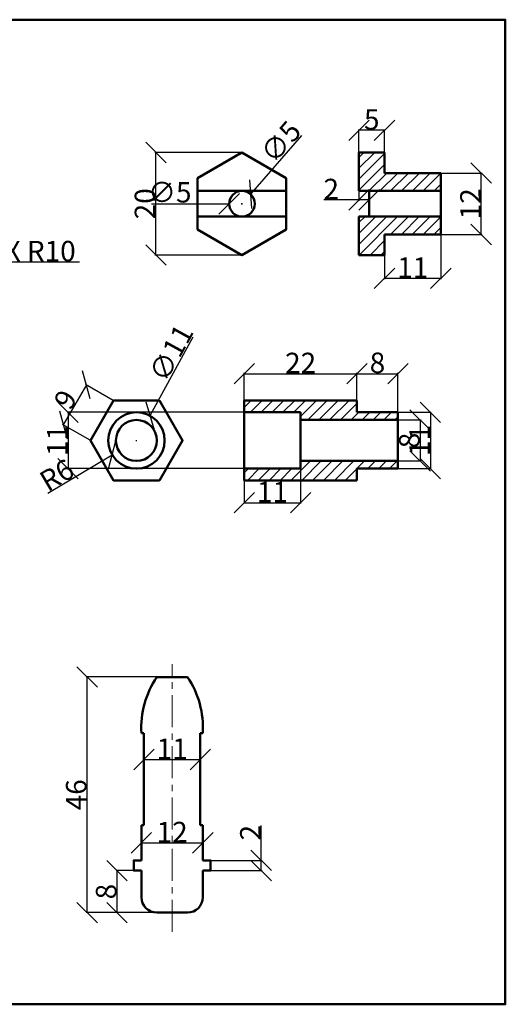
# Model space of a CAD drawing. Units: millimetres. Extents: x 4 to 224, y 3 to 195.
# Tile 2 of 2: x 129 to 224, y 3 to 195. Entities that reach past the tile are written whole.
import ezdxf

# ---------------------------------------------------------------- set-up
doc = ezdxf.new("R2010")
doc.units = ezdxf.units.MM
doc.header["$MEASUREMENT"] = 0
doc.linetypes.add('CENTER', pattern=[2, 1.25, -0.25, 0.25, -0.25])
for name, color, linetype, lineweight in [('M-CNTR', 1, 'CENTER', 18), ('M-DIMS', 2, 'Continuous', 25), ('M-HATC', 8, 'Continuous', 18), ('M-OUTL', 7, 'Continuous', 50)]:
    doc.layers.add(name, color=color, linetype=linetype, lineweight=lineweight)
doc.styles.get("Standard").update_dxf_attribs({"font": 'arial.ttf'})
doc.dimstyles.get("Standard").update_dxf_attribs({"dimtxt": 4, "dimasz": 4, "dimexe": 0.18, "dimexo": 0.0625, "dimgap": 0.09, "dimtad": 1, "dimdec": 0, "dimzin": 0, "dimdsep": 46, "dimtxsty": 'Standard', "dimblk": 'OBLIQUE', "dimcen": 0.09, "dimclre": 251, "dimadec": 0, "dimazin": 0, "dimtfac": 1, "dimtdec": 0, "dimtofl": 0, "dimtmove": 0, "dimatfit": 3, "dimfxl": 1, "dimtolj": 1, "dimtzin": 0, "dimarcsym": 0})

# ---------------------------------------------------------------- blocks, each defined once
blk = doc.blocks.new('_Oblique')
at = {"color": 0, "linetype": 'ByBlock', "lineweight": -2}
blk.add_line((-0.5, -0.5), (0.5, 0.5), dxfattribs=at)
blk = doc.blocks.new('*D10')
at = {"layer": 'Defpoints', "color": 0, "transparency": 16777216}
for p in [(156.03, 169.31), (172.83, 169.31), (172.83, 149.31)]:
    blk.add_point(p, dxfattribs=at)
at = {"layer": 'M-DIMS', "color": 0, "lineweight": -2, "transparency": 16777216}
for p, q in [((172.77, 169.31), (155.85, 169.31)), ((156.03, 149.31), (156.03, 169.31)), ((172.77, 149.31), (155.85, 149.31))]:
    blk.add_line(p, q, dxfattribs=at)
at = {"layer": 'M-DIMS', "color": 0, "lineweight": -2, "transparency": 16777216, "xscale": 4, "yscale": 4, "zscale": 4}
for p, rotation in [((156.03, 169.31), 90), ((156.03, 149.31), 270)]:
    blk.add_blockref('_Oblique', p, dxfattribs=dict(at, rotation=rotation))
at = {"layer": 'M-DIMS', "color": 0, "transparency": 16777216, "insert": (153.89, 159.31), "char_height": 4, "attachment_point": 5, "rotation": 90}
blk.add_mtext('\\A1;20', dxfattribs=at)
blk = doc.blocks.new('*D11')
at = {"layer": 'Defpoints', "color": 0, "transparency": 16777216}
for p in [(174.48, 161.19), (171.19, 157.43)]:
    blk.add_point(p, dxfattribs=at)
at = {"layer": 'M-DIMS', "color": 0, "lineweight": -2, "transparency": 16777216}
for p, q in [((184.47, 172.63), (174.48, 161.19)), ((172.74, 159.31), (172.92, 159.31)), ((172.83, 159.22), (172.83, 159.4))]:
    blk.add_line(p, q, dxfattribs=at)
at = {"layer": 'M-DIMS', "color": 0, "lineweight": -2, "transparency": 16777216, "xscale": 4, "yscale": 4, "zscale": 4, "rotation": 228.8599301228734}
blk.add_blockref('_Oblique', (174.48, 161.19), dxfattribs=at)
at = {"layer": 'M-DIMS', "color": 0, "transparency": 16777216, "insert": (180.42, 171.4), "char_height": 4, "attachment_point": 5, "rotation": 48.8599}
blk.add_mtext('\\A1;∅5', dxfattribs=at)
blk = doc.blocks.new('*D12')
at = {"layer": 'Defpoints', "color": 0, "transparency": 16777216}
for p in [(195.68, 173.66), (195.68, 169.31), (200.68, 169.31)]:
    blk.add_point(p, dxfattribs=at)
at = {"layer": 'M-DIMS', "color": 0, "lineweight": -2, "transparency": 16777216}
for p, q in [((195.68, 169.37), (195.68, 173.84)), ((200.68, 173.66), (195.68, 173.66)), ((200.68, 169.37), (200.68, 173.84))]:
    blk.add_line(p, q, dxfattribs=at)
at = {"layer": 'M-DIMS', "color": 0, "lineweight": -2, "transparency": 16777216, "xscale": 4, "yscale": 4, "zscale": 4, "rotation": 180}
blk.add_blockref('_Oblique', (195.68, 173.66), dxfattribs=at)
at = {"layer": 'M-DIMS', "color": 0, "lineweight": -2, "transparency": 16777216, "xscale": 4, "yscale": 4, "zscale": 4}
blk.add_blockref('_Oblique', (200.68, 173.66), dxfattribs=at)
at = {"layer": 'M-DIMS', "color": 0, "transparency": 16777216, "insert": (198.18, 175.78), "char_height": 4, "attachment_point": 5}
blk.add_mtext('\\A1;5', dxfattribs=at)
blk = doc.blocks.new('*D13')
at = {"layer": 'Defpoints', "color": 0, "transparency": 16777216}
for p in [(195.68, 161.81), (197.68, 161.81), (195.68, 160.09)]:
    blk.add_point(p, dxfattribs=at)
at = {"layer": 'M-DIMS', "color": 0, "lineweight": -2, "transparency": 16777216}
for p, q in [((195.68, 161.75), (195.68, 159.91)), ((197.68, 161.75), (197.68, 159.91)), ((195.68, 160.09), (188.85, 160.09)), ((197.68, 160.09), (195.68, 160.09))]:
    blk.add_line(p, q, dxfattribs=at)
at = {"layer": 'M-DIMS', "color": 0, "lineweight": -2, "transparency": 16777216, "xscale": 4, "yscale": 4, "zscale": 4, "rotation": 180}
blk.add_blockref('_Oblique', (195.68, 160.09), dxfattribs=at)
at = {"layer": 'M-DIMS', "color": 0, "lineweight": -2, "transparency": 16777216, "xscale": 4, "yscale": 4, "zscale": 4}
blk.add_blockref('_Oblique', (197.68, 160.09), dxfattribs=at)
at = {"layer": 'M-DIMS', "color": 0, "transparency": 16777216, "insert": (190.27, 162.19), "char_height": 4, "attachment_point": 5}
blk.add_mtext('\\A1;2', dxfattribs=at)
blk = doc.blocks.new('*D14')
at = {"layer": 'Defpoints', "color": 0, "transparency": 16777216}
for p in [(211.68, 153.31), (200.68, 149.31), (211.68, 144.77)]:
    blk.add_point(p, dxfattribs=at)
at = {"layer": 'M-DIMS', "color": 0, "lineweight": -2, "transparency": 16777216}
for p, q in [((211.68, 153.25), (211.68, 144.59)), ((200.68, 149.25), (200.68, 144.59)), ((200.68, 144.77), (211.68, 144.77))]:
    blk.add_line(p, q, dxfattribs=at)
at = {"layer": 'M-DIMS', "color": 0, "lineweight": -2, "transparency": 16777216, "xscale": 4, "yscale": 4, "zscale": 4, "rotation": 180}
blk.add_blockref('_Oblique', (200.68, 144.77), dxfattribs=at)
at = {"layer": 'M-DIMS', "color": 0, "lineweight": -2, "transparency": 16777216, "xscale": 4, "yscale": 4, "zscale": 4}
blk.add_blockref('_Oblique', (211.68, 144.77), dxfattribs=at)
at = {"layer": 'M-DIMS', "color": 0, "transparency": 16777216, "insert": (206.18, 146.86), "char_height": 4, "attachment_point": 5}
blk.add_mtext('\\A1;11', dxfattribs=at)
blk = doc.blocks.new('*D15')
at = {"layer": 'Defpoints', "color": 0, "transparency": 16777216}
for p in [(211.68, 165.31), (219.55, 165.31), (211.68, 153.31)]:
    blk.add_point(p, dxfattribs=at)
at = {"layer": 'M-DIMS', "color": 0, "lineweight": -2, "transparency": 16777216}
for p, q in [((211.75, 165.31), (219.73, 165.31)), ((219.55, 153.31), (219.55, 165.31)), ((211.75, 153.31), (219.73, 153.31))]:
    blk.add_line(p, q, dxfattribs=at)
at = {"layer": 'M-DIMS', "color": 0, "lineweight": -2, "transparency": 16777216, "xscale": 4, "yscale": 4, "zscale": 4}
for p, rotation in [((219.55, 165.31), 90), ((219.55, 153.31), 270)]:
    blk.add_blockref('_Oblique', p, dxfattribs=dict(at, rotation=rotation))
at = {"layer": 'M-DIMS', "color": 0, "transparency": 16777216, "insert": (217.45, 159.31), "char_height": 4, "attachment_point": 5, "rotation": 90}
blk.add_mtext('\\A1;12', dxfattribs=at)
blk = doc.blocks.new('*D16')
at = {"layer": 'Defpoints', "color": 0, "transparency": 16777216}
for p in [(147.73, 120.89), (137.95, 116.14), (143.23, 113.1)]:
    blk.add_point(p, dxfattribs=at)
at = {"layer": 'M-DIMS', "color": 0, "lineweight": -2, "transparency": 16777216}
for p, q in [((142.45, 123.94), (137.95, 116.14)), ((147.67, 120.92), (142.3, 124.03)), ((143.17, 113.13), (137.8, 116.23))]:
    blk.add_line(p, q, dxfattribs=at)
at = {"layer": 'M-DIMS', "color": 0, "lineweight": -2, "transparency": 16777216, "xscale": 4, "yscale": 4, "zscale": 4}
for p, rotation in [((142.45, 123.94), 60.00000000000002), ((137.95, 116.14), 240)]:
    blk.add_blockref('_Oblique', p, dxfattribs=dict(at, rotation=rotation))
at = {"layer": 'M-DIMS', "color": 0, "transparency": 16777216, "insert": (138.36, 121.1), "char_height": 4, "attachment_point": 5, "rotation": 60}
blk.add_mtext('\\A1;9', dxfattribs=at)
blk = doc.blocks.new('*D17')
at = {"layer": 'Defpoints', "color": 0, "transparency": 16777216}
for p in [(154.87, 117.92), (149.59, 108.27)]:
    blk.add_point(p, dxfattribs=at)
at = {"layer": 'M-DIMS', "color": 0, "lineweight": -2, "transparency": 16777216}
for p, q in [((163.26, 133.27), (154.87, 117.92)), ((152.14, 113.1), (152.32, 113.1)), ((152.23, 113.01), (152.23, 113.19))]:
    blk.add_line(p, q, dxfattribs=at)
at = {"layer": 'M-DIMS', "color": 0, "lineweight": -2, "transparency": 16777216, "xscale": 4, "yscale": 4, "zscale": 4, "rotation": 241.3177758891401}
blk.add_blockref('_Oblique', (154.87, 117.92), dxfattribs=at)
at = {"layer": 'M-DIMS', "color": 0, "transparency": 16777216, "insert": (159.01, 130.18), "char_height": 4, "attachment_point": 5, "rotation": 61.3178}
blk.add_mtext('\\A1;∅11', dxfattribs=at)
blk = doc.blocks.new('*D18')
at = {"layer": 'Defpoints', "color": 0, "transparency": 16777216}
for p in [(152.23, 113.1), (147.5, 110.29)]:
    blk.add_point(p, dxfattribs=at)
at = {"layer": 'M-DIMS', "color": 0, "lineweight": -2, "transparency": 16777216}
for p, q in [((152.14, 113.1), (152.32, 113.1)), ((152.23, 113.01), (152.23, 113.19)), ((134.91, 102.83), (147.5, 110.29))]:
    blk.add_line(p, q, dxfattribs=at)
at = {"layer": 'M-DIMS', "color": 0, "lineweight": -2, "transparency": 16777216, "xscale": 4, "yscale": 4, "zscale": 4, "rotation": 30.67031769012258}
blk.add_blockref('_Oblique', (147.5, 110.29), dxfattribs=at)
at = {"layer": 'M-DIMS', "color": 0, "transparency": 16777216, "insert": (136.68, 106.36), "char_height": 4, "attachment_point": 5, "rotation": 30.6703}
blk.add_mtext('\\A1;R6', dxfattribs=at)
blk = doc.blocks.new('*D19')
at = {"layer": 'Defpoints', "color": 0, "transparency": 16777216}
for p in [(195.29, 126.13), (173.29, 120.89), (195.29, 120.89)]:
    blk.add_point(p, dxfattribs=at)
at = {"layer": 'M-DIMS', "color": 0, "lineweight": -2, "transparency": 16777216}
for p, q in [((173.29, 120.95), (173.29, 126.31)), ((173.29, 126.13), (195.29, 126.13)), ((195.29, 120.95), (195.29, 126.31))]:
    blk.add_line(p, q, dxfattribs=at)
at = {"layer": 'M-DIMS', "color": 0, "lineweight": -2, "transparency": 16777216, "xscale": 4, "yscale": 4, "zscale": 4, "rotation": 180}
blk.add_blockref('_Oblique', (173.29, 126.13), dxfattribs=at)
at = {"layer": 'M-DIMS', "color": 0, "lineweight": -2, "transparency": 16777216, "xscale": 4, "yscale": 4, "zscale": 4}
blk.add_blockref('_Oblique', (195.29, 126.13), dxfattribs=at)
at = {"layer": 'M-DIMS', "color": 0, "transparency": 16777216, "insert": (184.29, 128.23), "char_height": 4, "attachment_point": 5}
blk.add_mtext('\\A1;22', dxfattribs=at)
blk = doc.blocks.new('*D20')
at = {"layer": 'Defpoints', "color": 0, "transparency": 16777216}
for p in [(203.29, 126.13), (195.29, 118.6), (203.29, 118.6)]:
    blk.add_point(p, dxfattribs=at)
at = {"layer": 'M-DIMS', "color": 0, "lineweight": -2, "transparency": 16777216}
for p, q in [((195.29, 118.66), (195.29, 126.31)), ((195.29, 126.13), (203.29, 126.13)), ((203.29, 118.66), (203.29, 126.31))]:
    blk.add_line(p, q, dxfattribs=at)
at = {"layer": 'M-DIMS', "color": 0, "lineweight": -2, "transparency": 16777216, "xscale": 4, "yscale": 4, "zscale": 4, "rotation": 180}
blk.add_blockref('_Oblique', (195.29, 126.13), dxfattribs=at)
at = {"layer": 'M-DIMS', "color": 0, "lineweight": -2, "transparency": 16777216, "xscale": 4, "yscale": 4, "zscale": 4}
blk.add_blockref('_Oblique', (203.29, 126.13), dxfattribs=at)
at = {"layer": 'M-DIMS', "color": 0, "transparency": 16777216, "insert": (199.29, 128.26), "char_height": 4, "attachment_point": 5}
blk.add_mtext('\\A1;8', dxfattribs=at)
blk = doc.blocks.new('*D21')
at = {"layer": 'Defpoints', "color": 0, "transparency": 16777216}
for p in [(203.29, 118.6), (203.29, 107.6), (209.63, 107.6)]:
    blk.add_point(p, dxfattribs=at)
at = {"layer": 'M-DIMS', "color": 0, "lineweight": -2, "transparency": 16777216}
for p, q in [((203.35, 118.6), (209.81, 118.6)), ((209.63, 118.6), (209.63, 107.6)), ((203.35, 107.6), (209.81, 107.6))]:
    blk.add_line(p, q, dxfattribs=at)
at = {"layer": 'M-DIMS', "color": 0, "lineweight": -2, "transparency": 16777216, "xscale": 4, "yscale": 4, "zscale": 4}
for p, rotation in [((209.63, 118.6), 90), ((209.63, 107.6), 270)]:
    blk.add_blockref('_Oblique', p, dxfattribs=dict(at, rotation=rotation))
at = {"layer": 'M-DIMS', "color": 0, "transparency": 16777216, "insert": (207.53, 113.1), "char_height": 4, "attachment_point": 5, "rotation": 90}
blk.add_mtext('\\A1;11', dxfattribs=at)
blk = doc.blocks.new('*D30')
at = {"layer": 'Defpoints', "color": 0, "transparency": 16777216}
for p in [(142.61, 66.92), (156.2, 66.92), (156.2, 20.92)]:
    blk.add_point(p, dxfattribs=at)
at = {"layer": 'M-DIMS', "color": 0, "lineweight": -2, "transparency": 16777216}
for p, q in [((156.14, 66.92), (142.43, 66.92)), ((142.61, 20.92), (142.61, 66.92)), ((156.14, 20.92), (142.43, 20.92))]:
    blk.add_line(p, q, dxfattribs=at)
at = {"layer": 'M-DIMS', "color": 0, "lineweight": -2, "transparency": 16777216, "xscale": 4, "yscale": 4, "zscale": 4}
for p, rotation in [((142.61, 66.92), 90), ((142.61, 20.92), 270)]:
    blk.add_blockref('_Oblique', p, dxfattribs=dict(at, rotation=rotation))
at = {"layer": 'M-DIMS', "color": 0, "transparency": 16777216, "insert": (140.47, 43.92), "char_height": 4, "attachment_point": 5, "rotation": 90}
blk.add_mtext('\\A1;46', dxfattribs=at)
blk = doc.blocks.new('*D31')
at = {"layer": 'Defpoints', "color": 0, "transparency": 16777216}
for p in [(148.44, 29.12), (151.7, 29.12), (156.2, 20.92)]:
    blk.add_point(p, dxfattribs=at)
at = {"layer": 'M-DIMS', "color": 0, "lineweight": -2, "transparency": 16777216}
for p, q in [((151.64, 29.12), (148.26, 29.12)), ((148.44, 20.92), (148.44, 29.12)), ((156.14, 20.92), (148.26, 20.92))]:
    blk.add_line(p, q, dxfattribs=at)
at = {"layer": 'M-DIMS', "color": 0, "lineweight": -2, "transparency": 16777216, "xscale": 4, "yscale": 4, "zscale": 4}
for p, rotation in [((148.44, 29.12), 90), ((148.44, 20.92), 270)]:
    blk.add_blockref('_Oblique', p, dxfattribs=dict(at, rotation=rotation))
at = {"layer": 'M-DIMS', "color": 0, "transparency": 16777216, "insert": (146.31, 25.02), "char_height": 4, "attachment_point": 5, "rotation": 90}
blk.add_mtext('\\A1;8', dxfattribs=at)
blk = doc.blocks.new('*D32')
at = {"layer": 'Defpoints', "color": 0, "transparency": 16777216}
for p in [(153.7, 50.38), (164.7, 50.81), (164.7, 50.38)]:
    blk.add_point(p, dxfattribs=at)
at = {"layer": 'M-DIMS', "color": 0, "lineweight": -2, "transparency": 16777216}
for p, q in [((153.7, 50.44), (153.7, 50.99)), ((153.7, 50.81), (164.7, 50.81)), ((164.7, 50.44), (164.7, 50.99))]:
    blk.add_line(p, q, dxfattribs=at)
at = {"layer": 'M-DIMS', "color": 0, "lineweight": -2, "transparency": 16777216, "xscale": 4, "yscale": 4, "zscale": 4, "rotation": 180}
blk.add_blockref('_Oblique', (153.7, 50.81), dxfattribs=at)
at = {"layer": 'M-DIMS', "color": 0, "lineweight": -2, "transparency": 16777216, "xscale": 4, "yscale": 4, "zscale": 4}
blk.add_blockref('_Oblique', (164.7, 50.81), dxfattribs=at)
at = {"layer": 'M-DIMS', "color": 0, "transparency": 16777216, "insert": (159.2, 52.91), "char_height": 4, "attachment_point": 5}
blk.add_mtext('\\A1;11', dxfattribs=at)
blk = doc.blocks.new('*D33')
at = {"layer": 'Defpoints', "color": 0, "transparency": 16777216}
for p in [(153.2, 34.54), (165.2, 34.54), (165.2, 34.54)]:
    blk.add_point(p, dxfattribs=at)
at = {"layer": 'M-DIMS', "color": 0, "lineweight": -2, "transparency": 16777216}
for p, q in [((153.2, 34.6), (153.2, 34.72)), ((165.2, 34.6), (165.2, 34.72)), ((153.2, 34.54), (165.2, 34.54))]:
    blk.add_line(p, q, dxfattribs=at)
at = {"layer": 'M-DIMS', "color": 0, "lineweight": -2, "transparency": 16777216, "xscale": 4, "yscale": 4, "zscale": 4, "rotation": 180}
blk.add_blockref('_Oblique', (153.2, 34.54), dxfattribs=at)
at = {"layer": 'M-DIMS', "color": 0, "lineweight": -2, "transparency": 16777216, "xscale": 4, "yscale": 4, "zscale": 4}
blk.add_blockref('_Oblique', (165.2, 34.54), dxfattribs=at)
at = {"layer": 'M-DIMS', "color": 0, "transparency": 16777216, "insert": (159.2, 36.64), "char_height": 4, "attachment_point": 5}
blk.add_mtext('\\A1;12', dxfattribs=at)
blk = doc.blocks.new('*D34')
at = {"layer": 'Defpoints', "color": 0, "transparency": 16777216}
for p in [(166.7, 31.12), (176.57, 31.12), (166.7, 29.12)]:
    blk.add_point(p, dxfattribs=at)
at = {"layer": 'M-DIMS', "color": 0, "lineweight": -2, "transparency": 16777216}
for p, q in [((176.57, 31.12), (176.57, 37.95)), ((166.76, 31.12), (176.75, 31.12)), ((176.57, 29.12), (176.57, 31.12)), ((166.76, 29.12), (176.75, 29.12))]:
    blk.add_line(p, q, dxfattribs=at)
at = {"layer": 'M-DIMS', "color": 0, "lineweight": -2, "transparency": 16777216, "xscale": 4, "yscale": 4, "zscale": 4}
for p, rotation in [((176.57, 31.12), 90), ((176.57, 29.12), 270)]:
    blk.add_blockref('_Oblique', p, dxfattribs=dict(at, rotation=rotation))
at = {"layer": 'M-DIMS', "color": 0, "transparency": 16777216, "insert": (174.47, 36.53), "char_height": 4, "attachment_point": 5, "rotation": 90}
blk.add_mtext('\\A1;2', dxfattribs=at)
blk = doc.blocks.new('*D35')
at = {"layer": 'Defpoints', "color": 0, "transparency": 16777216}
for p in [(184.29, 117.1), (184.29, 109.1), (207.64, 109.1)]:
    blk.add_point(p, dxfattribs=at)
at = {"layer": 'M-DIMS', "color": 251, "lineweight": -2, "transparency": 16777216}
for p, q in [((184.35, 117.1), (207.82, 117.1)), ((184.35, 109.1), (207.82, 109.1))]:
    blk.add_line(p, q, dxfattribs=at)
at = {"layer": 'M-DIMS', "color": 0, "lineweight": -2, "transparency": 16777216}
blk.add_line((207.64, 117.1), (207.64, 109.1), dxfattribs=at)
at = {"layer": 'M-DIMS', "color": 0, "lineweight": -2, "transparency": 16777216, "xscale": 4, "yscale": 4, "zscale": 4}
for p, rotation in [((207.64, 117.1), 90), ((207.64, 109.1), 270)]:
    blk.add_blockref('_Oblique', p, dxfattribs=dict(at, rotation=rotation))
at = {"layer": 'M-DIMS', "color": 0, "transparency": 16777216, "insert": (205.51, 113.1), "char_height": 4, "attachment_point": 5, "rotation": 90}
blk.add_mtext('\\A1;8', dxfattribs=at)
blk = doc.blocks.new('*D36')
at = {"layer": 'Defpoints', "color": 0, "transparency": 16777216}
for p in [(173.29, 107.6), (184.29, 107.6), (184.29, 100.95)]:
    blk.add_point(p, dxfattribs=at)
at = {"layer": 'M-DIMS', "color": 251, "lineweight": -2, "transparency": 16777216}
for p, q in [((173.29, 107.54), (173.29, 100.77)), ((184.29, 107.54), (184.29, 100.77))]:
    blk.add_line(p, q, dxfattribs=at)
at = {"layer": 'M-DIMS', "color": 0, "lineweight": -2, "transparency": 16777216}
blk.add_line((173.29, 100.95), (184.29, 100.95), dxfattribs=at)
at = {"layer": 'M-DIMS', "color": 0, "lineweight": -2, "transparency": 16777216, "xscale": 4, "yscale": 4, "zscale": 4, "rotation": 180}
blk.add_blockref('_Oblique', (173.29, 100.95), dxfattribs=at)
at = {"layer": 'M-DIMS', "color": 0, "lineweight": -2, "transparency": 16777216, "xscale": 4, "yscale": 4, "zscale": 4}
blk.add_blockref('_Oblique', (184.29, 100.95), dxfattribs=at)
at = {"layer": 'M-DIMS', "color": 0, "transparency": 16777216, "insert": (178.79, 103.05), "char_height": 4, "attachment_point": 5}
blk.add_mtext('\\A1;11', dxfattribs=at)
blk = doc.blocks.new('*D39')
at = {"layer": 'Defpoints', "color": 0, "transparency": 16777216}
for p in [(173.29, 118.6), (138.88, 107.6), (173.29, 107.6)]:
    blk.add_point(p, dxfattribs=at)
at = {"layer": 'M-DIMS', "color": 251, "lineweight": -2, "transparency": 16777216}
for p, q in [((173.23, 118.6), (138.7, 118.6)), ((173.23, 107.6), (138.7, 107.6))]:
    blk.add_line(p, q, dxfattribs=at)
at = {"layer": 'M-DIMS', "color": 0, "lineweight": -2, "transparency": 16777216}
blk.add_line((138.88, 118.6), (138.88, 107.6), dxfattribs=at)
at = {"layer": 'M-DIMS', "color": 0, "lineweight": -2, "transparency": 16777216, "xscale": 4, "yscale": 4, "zscale": 4}
for p, rotation in [((138.88, 118.6), 90), ((138.88, 107.6), 270)]:
    blk.add_blockref('_Oblique', p, dxfattribs=dict(at, rotation=rotation))
at = {"layer": 'M-DIMS', "color": 0, "transparency": 16777216, "insert": (136.78, 113.1), "char_height": 4, "attachment_point": 5, "rotation": 90}
blk.add_mtext('\\A1;11', dxfattribs=at)
blk = doc.blocks.new('*D42')
at = {"layer": 'Defpoints', "color": 0, "transparency": 16777216}
for p in [(104.72, 147.94), (114.72, 147.94)]:
    blk.add_point(p, dxfattribs=at)
at = {"layer": 'M-DIMS', "color": 251, "lineweight": -2, "transparency": 16777216}
for p, q in [((104.72, 147.85), (104.72, 148.03)), ((104.63, 147.94), (104.81, 147.94))]:
    blk.add_line(p, q, dxfattribs=at)
at = {"layer": 'M-DIMS', "color": 0, "lineweight": -2, "transparency": 16777216}
blk.add_line((141.11, 147.93), (114.72, 147.94), dxfattribs=at)
at = {"layer": 'M-DIMS', "color": 0, "lineweight": -2, "transparency": 16777216, "xscale": 4, "yscale": 4, "zscale": 4, "rotation": 179.9762165209119}
blk.add_blockref('_Oblique', (114.72, 147.94), dxfattribs=at)
at = {"layer": 'M-DIMS', "color": 0, "transparency": 16777216, "insert": (131.91, 150.07), "char_height": 4, "attachment_point": 5, "rotation": 359.9762}
blk.add_mtext('\\A1;2X R10', dxfattribs=at)
blk = doc.blocks.new('*D44')
at = {"layer": 'Defpoints', "color": 0, "transparency": 16777216}
for p in [(170.33, 159.31), (175.33, 159.31)]:
    blk.add_point(p, dxfattribs=at)
at = {"layer": 'M-DIMS', "color": 0, "lineweight": -2, "transparency": 16777216}
blk.add_line((155.15, 159.32), (170.33, 159.31), dxfattribs=at)
at = {"layer": 'M-DIMS', "color": 251, "lineweight": -2, "transparency": 16777216}
for p, q in [((172.74, 159.31), (172.92, 159.31)), ((172.83, 159.22), (172.83, 159.4))]:
    blk.add_line(p, q, dxfattribs=at)
at = {"layer": 'M-DIMS', "color": 0, "lineweight": -2, "transparency": 16777216, "xscale": 4, "yscale": 4, "zscale": 4, "rotation": 359.9645682944653}
blk.add_blockref('_Oblique', (170.33, 159.31), dxfattribs=at)
at = {"layer": 'M-DIMS', "color": 0, "transparency": 16777216, "insert": (158.74, 161.56), "char_height": 4, "attachment_point": 5, "rotation": 359.9646}
blk.add_mtext('\\A1;∅5', dxfattribs=at)

msp = doc.modelspace()

# ---------------------------------------------------------------- hatches: boundary and pattern name
at = {"layer": 'M-HATC'}
h = msp.add_hatch(dxfattribs=at)
h.set_pattern_fill('ANSI31', color=256, scale=12)
h.set_pattern_definition([(45, (-14.3302, 24.1046), (-1.06066, 1.06066), [])])
h.paths.add_polyline_path([(211.6829, 161.8085), (211.6829, 165.3085), (200.6829, 165.3085), (200.6829, 169.3085), (195.6829, 169.3085), (195.6829, 161.8085)])
h.paths.add_polyline_path([(211.6829, 153.3085), (211.6829, 156.8085), (195.6829, 156.8085), (195.6829, 149.3085), (200.6829, 149.3085), (200.6829, 153.3085)])
h = msp.add_hatch(dxfattribs=at)
h.set_pattern_fill('ANSI31', color=256, scale=12)
h.set_pattern_definition([(45, (-18.809, 3.8051), (-1.06066, 1.06066), [])])
h.paths.add_polyline_path([(203.289, 117.098), (203.289, 118.598), (195.289, 118.598), (195.289, 120.8922), (173.289, 120.8922), (173.289, 118.598), (184.289, 118.598), (184.289, 117.098)])
h.paths.add_polyline_path([(195.289, 105.3037), (195.289, 107.598), (203.289, 107.598), (203.289, 109.098), (184.289, 109.098), (184.289, 107.598), (173.289, 107.598), (173.289, 105.3037)])

# ---------------------------------------------------------------- linework, layer by layer
at = {"layer": 'M-CNTR', "ltscale": 5}
msp.add_line((159.198, 17.1404), (159.198, 69.4089), dxfattribs=at)
at = {"layer": 'M-OUTL'}
for p, q in [((195.6829, 169.3085), (195.6829, 161.8085)), ((195.6829, 169.3085), (200.6829, 169.3085)), ((200.6829, 165.3085), (200.6829, 169.3085)), ((200.6829, 165.3085), (211.6829, 165.3085)), ((211.6829, 153.3085), (211.6829, 165.3085)), ((164.1741, 161.8085), (181.4946, 161.8085)), ((195.6829, 161.8085), (211.6829, 161.8085)), ((197.6829, 161.8085), (197.6829, 156.8085)), ((164.1741, 156.8085), (181.4946, 156.8085)), ((195.6829, 156.8085), (211.6829, 156.8085)), ((195.6829, 156.8085), (195.6829, 149.3085)), ((200.6829, 149.3085), (200.6829, 153.3085)), ((200.6829, 153.3085), (211.6829, 153.3085)), ((195.6829, 149.3085), (200.6829, 149.3085)), ((173.289, 120.8922), (173.289, 105.3037)), ((173.289, 120.8922), (195.289, 120.8922)), ((195.289, 118.598), (195.289, 120.8922)), ((173.289, 118.598), (184.289, 118.598)), ((184.289, 118.598), (184.289, 107.598)), ((195.289, 118.598), (203.289, 118.598)), ((203.289, 118.598), (203.289, 107.598)), ((184.289, 117.098), (203.289, 117.098)), ((184.289, 109.098), (203.289, 109.098)), ((173.289, 107.598), (184.289, 107.598)), ((195.289, 107.598), (203.289, 107.598)), ((195.289, 105.3037), (195.289, 107.598)), ((173.289, 105.3037), (195.289, 105.3037)), ((156.198, 66.9169), (162.198, 66.9169)), ((153.198, 55.9669), (153.698, 55.9669)), ((153.698, 37.9669), (153.698, 55.9669)), ((164.698, 37.9669), (164.698, 55.9669)), ((164.698, 55.9669), (165.198, 55.9669)), ((153.198, 31.1169), (153.198, 37.9669)), ((153.198, 37.9669), (153.698, 37.9669)), ((164.698, 37.9669), (165.198, 37.9669)), ((165.198, 31.1169), (165.198, 37.9669)), ((153.198, 23.9169), (153.198, 29.1169)), ((165.198, 23.9169), (165.198, 29.1169)), ((156.198, 20.9169), (162.198, 20.9169))]:
    msp.add_line(p, q, dxfattribs=at)
for points in [[(3.7754, 195.2521), (224.2583, 195.2521), (224.2583, 3.0162), (3.7754, 3.0162)], [(181.4946, 164.3085), (172.8344, 169.3085), (164.1741, 164.3085), (164.1741, 154.3085), (172.8344, 149.3085), (181.4946, 154.3085)], [(147.7259, 120.8922), (143.2259, 113.098), (147.7259, 105.3037), (156.7259, 105.3037), (161.2259, 113.098), (156.7259, 120.8922)]]:
    msp.add_lwpolyline(points, close=True, dxfattribs=at)
for points in [[(153.198, 29.1169), (151.698, 29.1169), (151.698, 31.1169), (153.198, 31.1169)], [(165.198, 31.1169), (166.698, 31.1169), (166.698, 29.1169), (165.198, 29.1169)]]:
    msp.add_lwpolyline(points, dxfattribs=at)
for centre, radius in [((172.8344, 159.3085), 2.5), ((152.2259, 113.098), 5.5), ((152.2259, 113.098), 4)]:
    msp.add_circle(centre, radius, dxfattribs=at)
for centre, radius, start, end in [((171.1723, 56.9284), 18, 146.294997, 183.061983), ((147.2237, 56.9284), 18, 356.938017, 33.705003), ((156.198, 23.9169), 3, 180, 270), ((162.198, 23.9169), 3, 270, 0)]:
    msp.add_arc(centre, radius, start, end, dxfattribs=at)

# ---------------------------------------------------------------- dimensions: what is measured, and where the dimension line sits
at = {"layer": 'M-DIMS'}
for base, p1, p2, override, picture, middle in [((195.6829, 173.6583), (200.6829, 169.3085), (195.6829, 169.3085), {"dimclrd": 0, "dimclre": 0, "dimclrt": 0}, '*D12', (198.1829, 175.7824)), ((195.6829, 160.0937), (197.6829, 161.8085), (195.6829, 161.8085), {"dimclrd": 0, "dimclre": 0, "dimclrt": 0}, '*D13', (190.2682, 162.1918)), ((211.6829, 144.766), (200.6829, 149.3085), (211.6829, 153.3085), {"dimclrd": 0, "dimclre": 0, "dimclrt": 0}, '*D14', (206.1829, 146.8641)), ((195.289, 126.1293), (173.289, 120.8922), (195.289, 120.8922), {"dimclrd": 0, "dimclre": 0, "dimclrt": 0}, '*D19', (184.289, 128.2275)), ((203.289, 126.1293), (195.289, 118.598), (203.289, 118.598), {"dimclrd": 0, "dimclre": 0, "dimclrt": 0}, '*D20', (199.289, 128.2616)), ((184.289, 100.9537), (173.289, 107.598), (184.289, 107.598), {"dimdec": 0, "dimlfac": 1, "dimrnd": 0, "dimzin": 0, "dimdsep": 46, "dimlunit": 2}, '*D36', (178.789, 103.0519)), ((164.698, 50.8078), (153.698, 50.3791), (164.698, 50.3791), {"dimclrd": 0, "dimclre": 0, "dimclrt": 0}, '*D32', (159.198, 52.9059)), ((165.198, 34.5419), (153.198, 34.5419), (165.198, 34.5419), {"dimclrd": 0, "dimclre": 0, "dimclrt": 0}, '*D33', (159.198, 36.6401))]:
    dim = msp.add_linear_dim(base=base, p1=p1, p2=p2, dimstyle='Standard', override=override, dxfattribs=at)
    dim.commit()
    dim.dimension.update_dxf_attribs({"geometry": picture, "text_midpoint": middle})
for p1, p2, picture, middle in [((171.1896, 157.4257), (174.4791, 161.1912), '*D11', (180.4155, 171.3977)), ((149.5862, 108.2728), (154.8657, 117.9231), '*D17', (159.0138, 130.1812))]:
    dim = msp.add_diameter_dim_2p(p1=p1, p2=p2, dimstyle='Standard', override={"dimclrd": 0, "dimclre": 0, "dimclrt": 0}, dxfattribs=at)
    dim.commit()
    dim.dimension.update_dxf_attribs({"geometry": picture, "text_midpoint": middle})
for base, p1, p2, override, picture, middle in [((156.0264, 169.3085), (172.8344, 149.3085), (172.8344, 169.3085), {"dimclrd": 0, "dimclre": 0, "dimclrt": 0}, '*D10', (153.8941, 159.3085)), ((219.551, 165.3085), (211.6829, 153.3085), (211.6829, 165.3085), {"dimclrd": 0, "dimclre": 0, "dimclrt": 0}, '*D15', (217.4528, 159.3085)), ((138.8759, 107.598), (173.289, 118.598), (173.289, 107.598), {"dimdec": 0, "dimlfac": 1, "dimrnd": 0, "dimzin": 0, "dimdsep": 46, "dimlunit": 2}, '*D39', (136.7777, 113.098)), ((209.6328, 107.598), (203.289, 118.598), (203.289, 107.598), {"dimclrd": 0, "dimclre": 0, "dimclrt": 0}, '*D21', (207.5346, 113.098)), ((207.639, 109.098), (184.289, 117.098), (184.289, 109.098), {"dimdec": 0, "dimlfac": 1, "dimrnd": 0, "dimzin": 0, "dimdsep": 46, "dimlunit": 2}, '*D35', (205.5067, 113.098)), ((142.6071, 66.9169), (156.198, 20.9169), (156.198, 66.9169), {"dimclrd": 0, "dimclre": 0, "dimclrt": 0}, '*D30', (140.4748, 43.9169)), ((176.5653, 31.1169), (166.698, 29.1169), (166.698, 31.1169), {"dimclrd": 0, "dimclre": 0, "dimclrt": 0}, '*D34', (174.4671, 36.5316)), ((148.4411, 29.1169), (156.198, 20.9169), (151.698, 29.1169), {"dimclrd": 0, "dimclre": 0, "dimclrt": 0}, '*D31', (146.3088, 25.0169))]:
    dim = msp.add_linear_dim(base=base, p1=p1, p2=p2, angle=90, dimstyle='Standard', override=override, dxfattribs=at)
    dim.commit()
    dim.dimension.update_dxf_attribs({"geometry": picture, "text_midpoint": middle})
dim = msp.add_diameter_dim_2p(p1=(175.3344, 159.3069), p2=(170.3344, 159.31), dimstyle='Standard', override={"dimdec": 0, "dimlfac": 1, "dimrnd": 0, "dimzin": 0, "dimdsep": 46, "dimlunit": 2}, dxfattribs=at)
dim.commit()
dim.dimension.update_dxf_attribs({"geometry": '*D44', "text_midpoint": (158.7423, 159.3172), "dimtype": 163})
dim = msp.add_radius_dim(center=(104.7199, 147.9442), mpoint=(114.7199, 147.94), text='2X <>', dimstyle='Standard', override={"dimdec": 0, "dimlfac": 1, "dimrnd": 0, "dimzin": 0, "dimdsep": 46, "dimlunit": 2}, dxfattribs=at)
dim.commit()
dim.dimension.update_dxf_attribs({"geometry": '*D42', "text_midpoint": (131.9145, 150.0652)})
dim = msp.add_aligned_dim(p1=(147.7259, 120.8922), p2=(143.2259, 113.098), distance=-6.0873, dimstyle='Standard', override={"dimclrd": 0, "dimclre": 0, "dimclrt": 0}, dxfattribs=at)
dim.commit()
dim.dimension.update_dxf_attribs({"geometry": '*D16', "text_midpoint": (138.3576, 121.1049)})
dim = msp.add_radius_dim(center=(152.22593, 113.09796), mpoint=(147.49529, 110.29242), dimstyle='Standard', override={"dimclrd": 0, "dimclre": 0, "dimclrt": 0}, dxfattribs=at)
dim.commit()
dim.dimension.update_dxf_attribs({"geometry": '*D18', "text_midpoint": (136.67648, 106.35534)})

doc.saveas('drawing.dxf')
